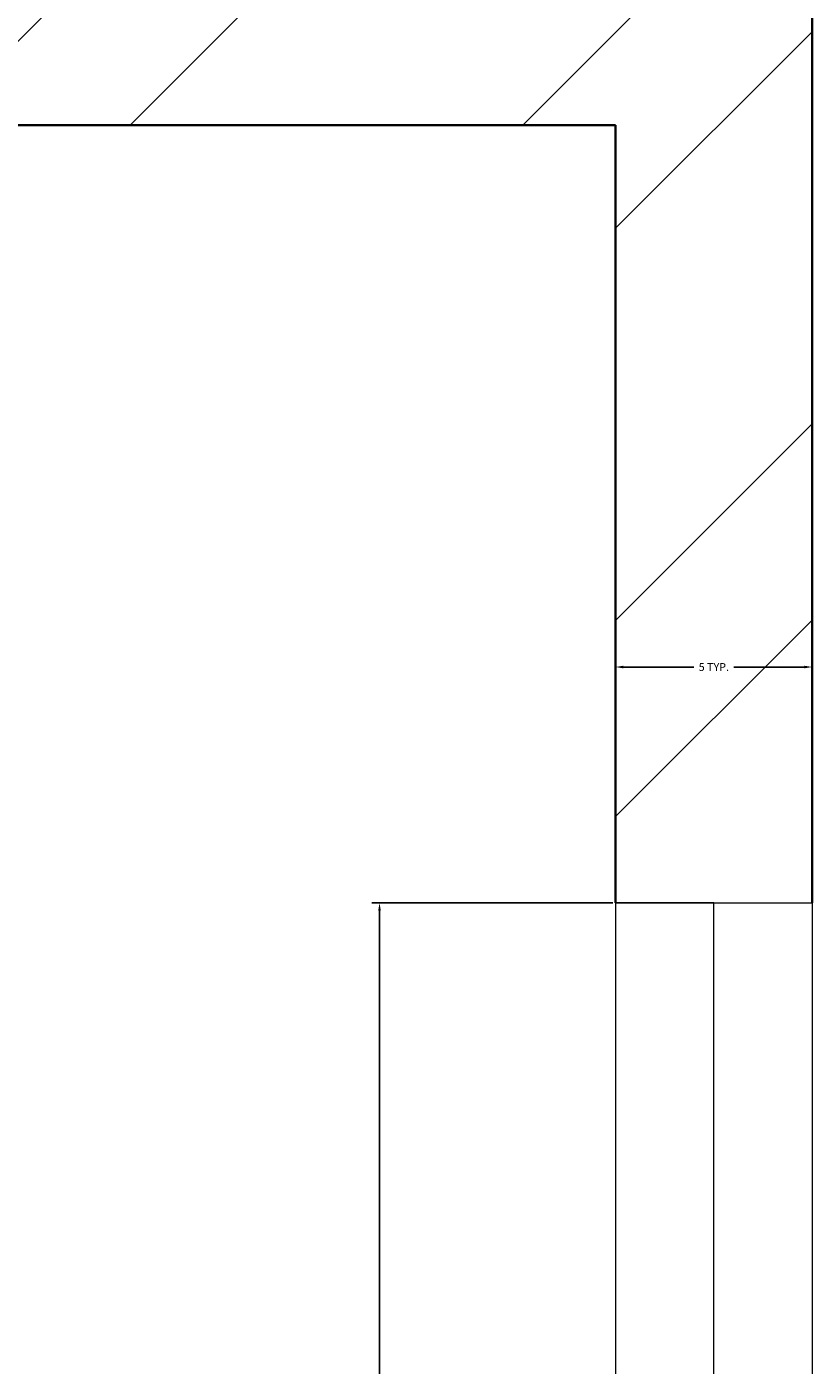
# Model space of a CAD drawing. Units: inches. Extents: x 2168 to 3056, y 1130 to 2629.
# Tile 20 of 42: x 2846 to 2864, y 2048 to 2079. Entities that reach past the tile are written whole.
import ezdxf

# ---------------------------------------------------------------- set-up
doc = ezdxf.new("R2010")
doc.units = ezdxf.units.IN
for name, color, linetype, lineweight in [('A-ANNO-DIMS', 2, 'Continuous', 18), ('A-GLAZ', 201, 'Continuous', 18), ('A-WALL', 7, 'Continuous', 35)]:
    doc.layers.add(name, color=color, linetype=linetype, lineweight=lineweight)
doc.layers.add('A-WALL-PATT', color=143, linetype='Continuous', lineweight=13, true_color=0x7aafdf)
doc.styles.get("Standard").update_dxf_attribs({"font": 'arial.ttf'})
doc.dimstyles.get("Standard").update_dxf_attribs({"dimtxt": 0.18, "dimasz": 0.18, "dimexe": 0.18, "dimexo": 0.0625, "dimgap": 0.09, "dimtad": 0, "dimtih": 1, "dimtoh": 1, "dimdec": 4, "dimzin": 0, "dimdsep": 46, "dimtxsty": 'Standard', "dimcen": 0.09, "dimadec": 0, "dimazin": 0, "dimtfac": 1, "dimtdec": 4, "dimtofl": 0, "dimtmove": 0, "dimatfit": 3, "dimfxl": 1, "dimtolj": 1, "dimtzin": 0, "dimarcsym": 0})

# ---------------------------------------------------------------- blocks, each defined once
blk = doc.blocks.new('WIN-36')
for p, q in [((2.25, 36), (0, 36)), ((0, 36), (4.5, 36)), ((0, 36), (0, 0)), ((2.25, 0), (2.25, 36)), ((4.5, 36), (4.5, 0))]:
    blk.add_line(p, q)
blk = doc.blocks.new('*D36')
at = {"layer": 'A-ANNO-DIMS', "color": 0, "lineweight": -2, "transparency": 16777216}
for p, q in [((2859.733, 2058.577), (2854.216, 2058.577)), ((2854.396, 2058.397), (2854.396, 2040.761)), ((2854.396, 2022.757), (2854.396, 2040.394)), ((2859.733, 2022.577), (2854.216, 2022.577))]:
    blk.add_line(p, q, dxfattribs=at)
at = {"layer": 'A-ANNO-DIMS', "color": 0, "transparency": 16777216}
for points in [[(2854.366, 2058.397), (2854.426, 2058.397), (2854.396, 2058.577)], [(2854.366, 2022.757), (2854.426, 2022.757), (2854.396, 2022.577)]]:
    blk.add_solid(points, dxfattribs=at)
at = {"layer": 'Defpoints', "color": 0, "transparency": 16777216}
for p in [(2854.396, 2058.577), (2859.796, 2058.577), (2859.796, 2022.577)]:
    blk.add_point(p, dxfattribs=at)
at = {"layer": 'A-ANNO-DIMS', "color": 0, "transparency": 16777216, "insert": (2854.396, 2040.577), "char_height": 0.18, "attachment_point": 5}
blk.add_mtext('\\A1;WINDOW 36 TYP.', dxfattribs=at)
blk = doc.blocks.new('*D37')
at = {"layer": 'A-ANNO-DIMS', "color": 0, "lineweight": -2, "transparency": 16777216}
for p, q in [((2859.796, 2058.64), (2859.796, 2064.157)), ((2864.296, 2058.64), (2864.296, 2064.157)), ((2859.976, 2063.977), (2861.588, 2063.977)), ((2864.116, 2063.977), (2862.504, 2063.977))]:
    blk.add_line(p, q, dxfattribs=at)
at = {"layer": 'A-ANNO-DIMS', "color": 0, "transparency": 16777216}
for points in [[(2859.976, 2064.007), (2859.976, 2063.947), (2859.796, 2063.977)], [(2864.116, 2064.007), (2864.116, 2063.947), (2864.296, 2063.977)]]:
    blk.add_solid(points, dxfattribs=at)
at = {"layer": 'Defpoints', "color": 0, "transparency": 16777216}
for p in [(2864.296, 2063.977), (2859.796, 2058.577), (2864.296, 2058.577)]:
    blk.add_point(p, dxfattribs=at)
at = {"layer": 'A-ANNO-DIMS', "color": 0, "transparency": 16777216, "insert": (2862.046, 2063.977), "char_height": 0.18, "attachment_point": 5}
blk.add_mtext('\\A1;5 TYP.', dxfattribs=at)

msp = doc.modelspace()

# ---------------------------------------------------------------- hatches: boundary and pattern name
at = {"layer": 'A-WALL-PATT'}
h = msp.add_hatch(dxfattribs=at)
h.set_pattern_fill('ANSI32', color=256)
h.paths.add_polyline_path([(2463.796, 2409.389), (2467.387, 2409.389), (2467.387, 2413.889), (2454.768, 2413.889), (2454.768, 2411.639), (2454.768, 2409.389), (2459.296, 2409.389), (2459.296, 2265.389), (2455.644, 2265.389), (2455.644, 2260.889), (2467.349, 2260.889), (2467.349, 2263.139), (2467.349, 2265.389), (2463.796, 2265.389)])
h.paths.add_polyline_path([(2431.596, 2413.889), (2409.647, 2413.889), (2409.647, 2409.389), (2431.596, 2409.389), (2431.596, 2411.639)])
h.paths.add_polyline_path([(2349.647, 2413.889), (2331.796, 2413.889), (2331.796, 2362.671), (2336.296, 2362.671), (2336.296, 2409.389), (2349.647, 2409.389), (2349.647, 2411.639)])
h.paths.add_polyline_path([(2634.149, 2411.639), (2634.149, 2413.889), (2562.293, 2413.889), (2562.293, 2409.389), (2595.796, 2409.389), (2595.796, 2280.309), (2595.826, 2280.309), (2595.826, 2265.389), (2499.91, 2265.389), (2499.91, 2260.889), (2550.796, 2260.889), (2550.796, 2117.308), (2555.296, 2117.308), (2555.296, 2168.08), (2571.93, 2168.08), (2571.93, 2176.889), (2559.796, 2176.889), (2559.796, 2256.389), (2640.796, 2256.389), (2640.796, 2176.889), (2626.428, 2176.889), (2626.428, 2168.08), (2645.296, 2168.08), (2645.296, 2116.637), (2649.796, 2116.637), (2649.796, 2260.889), (2691.251, 2260.889), (2691.251, 2263.139), (2691.251, 2265.389), (2670.655, 2265.389), (2670.655, 2265.365), (2600.296, 2265.365), (2600.296, 2280.258), (2600.296, 2409.389), (2634.149, 2409.389)])
h.paths.add_polyline_path([(2600.296, 2473.889), (2612.84, 2473.889), (2612.84, 2478.389), (2572.636, 2478.389), (2572.636, 2473.889), (2595.796, 2473.889), (2595.796, 2413.889), (2600.296, 2413.889)])
h.paths.add_polyline_path([(2535.796, 2473.889), (2548.636, 2473.889), (2548.636, 2478.389), (2531.396, 2478.389), (2531.396, 2413.889), (2521.6, 2413.889), (2521.6, 2409.389), (2539.239, 2409.389), (2539.239, 2411.639), (2539.239, 2413.889), (2535.796, 2413.889)])
h.paths.add_polyline_path([(2664.796, 2478.389), (2636.84, 2478.389), (2636.84, 2473.889), (2660.296, 2473.889), (2660.296, 2413.889), (2656.165, 2413.889), (2656.165, 2409.389), (2671.684, 2409.389), (2671.684, 2411.639), (2671.684, 2413.889), (2664.796, 2413.889)])
h.paths.add_polyline_path([(2705.942, 2413.889), (2695.684, 2413.889), (2695.684, 2409.389), (2705.942, 2409.389)])
h.paths.add_polyline_path([(2741.35, 2413.889), (2728.733, 2413.889), (2728.733, 2411.639), (2728.733, 2409.389), (2732.296, 2409.389), (2732.296, 2265.389), (2725.733, 2265.389), (2725.733, 2260.889), (2740.917, 2260.889), (2740.917, 2263.139), (2740.917, 2265.389), (2736.796, 2265.389), (2736.796, 2409.389), (2741.35, 2409.389)])
h.paths.add_polyline_path([(2785.655, 2413.889), (2764.546, 2413.889), (2764.486, 2409.389), (2785.655, 2409.389), (2785.655, 2411.639)])
h.paths.add_polyline_path([(2864.296, 2413.889), (2845.655, 2413.889), (2845.655, 2409.389), (2859.796, 2409.389), (2859.796, 2368.425), (2864.296, 2368.425)])
h.paths.add_polyline_path([(2864.296, 2308.425), (2862.046, 2308.425), (2859.796, 2308.425), (2859.796, 2265.389), (2774.483, 2265.389), (2774.483, 2263.139), (2774.483, 2260.889), (2781.796, 2260.889), (2781.796, 2226.654), (2786.296, 2226.654), (2786.296, 2260.889), (2859.796, 2260.889), (2859.796, 2241.352), (2864.296, 2241.352)])
h.paths.add_polyline_path([(2864.296, 2217.352), (2862.046, 2217.352), (2859.796, 2217.352), (2859.796, 2200.889), (2786.296, 2200.889), (2786.296, 2205.931), (2784.046, 2205.931), (2781.796, 2205.931), (2781.796, 2150.974), (2786.296, 2150.974), (2786.296, 2161.889), (2859.796, 2161.889), (2859.796, 2144.419), (2864.296, 2144.419)])
h.paths.add_polyline_path([(2859.796, 2196.389), (2859.796, 2166.389), (2786.296, 2166.389), (2786.296, 2196.389)], flags=16)
h.paths.add_polyline_path([(2864.296, 2108.419), (2862.046, 2108.419), (2859.796, 2108.419), (2859.796, 2080.889), (2786.296, 2080.889), (2786.296, 2111.993), (2781.796, 2111.993), (2781.796, 2080.889), (2649.796, 2080.889), (2649.796, 2086.036), (2647.546, 2086.036), (2645.296, 2086.036), (2645.296, 2071.739), (2649.796, 2071.739), (2649.796, 2076.389), (2781.796, 2076.389), (2781.796, 2041.792), (2786.296, 2041.792), (2786.296, 2076.389), (2859.796, 2076.389), (2859.796, 2058.577), (2864.296, 2058.577)])
h.paths.add_polyline_path([(2864.296, 2022.577), (2859.796, 2022.577), (2859.796, 1992.389), (2786.296, 1992.389), (2786.296, 1999.573), (2781.796, 1999.573), (2781.796, 1848.085), (2784.046, 1848.085), (2786.296, 1848.085), (2786.296, 1851.389), (2859.796, 1851.389), (2859.796, 1838.258), (2864.296, 1838.258)], flags=17)
h.paths.add_polyline_path([(2859.796, 1987.889), (2859.796, 1855.889), (2786.296, 1855.889), (2786.296, 1987.889)], flags=16)
h.paths.add_polyline_path([(2823.046, 1987.889), (2841.421, 1921.889), (2823.046, 1855.889)], flags=0)
h.paths.add_polyline_path([(2864.296, 1814.258), (2859.796, 1814.258), (2859.796, 1791.389), (2786.296, 1791.389), (2786.296, 1825.658), (2784.046, 1825.658), (2781.796, 1825.658), (2781.796, 1791.389), (2720.155, 1791.389), (2720.155, 1791.265), (2649.796, 1791.265), (2649.796, 1806.159), (2649.796, 2038.983), (2647.546, 2038.983), (2645.296, 2038.983), (2645.296, 1783.925), (2649.796, 1783.925), (2649.796, 1786.889), (2781.796, 1786.889), (2781.796, 1746.789), (2786.296, 1746.789), (2786.296, 1786.889), (2859.796, 1786.889), (2859.796, 1770.083), (2864.296, 1770.083)])
h.paths.add_polyline_path([(2864.296, 1734.083), (2862.046, 1734.083), (2859.796, 1734.083), (2859.796, 1705.889), (2786.296, 1705.889), (2786.296, 1714.166), (2781.796, 1714.166), (2781.796, 1660.527), (2786.296, 1660.527), (2786.296, 1666.889), (2859.796, 1666.889), (2859.796, 1648.342), (2864.296, 1648.342)])
h.paths.add_polyline_path([(2786.296, 1701.389), (2859.796, 1701.389), (2859.796, 1671.389), (2786.296, 1671.389)], flags=16)
h.paths.add_polyline_path([(2649.796, 1756.576), (2647.546, 1756.576), (2645.296, 1756.576), (2645.296, 1606.889), (2555.296, 1606.889), (2555.296, 1749.513), (2553.046, 1749.513), (2550.796, 1749.513), (2550.796, 1606.889), (2503.006, 1606.889), (2503.006, 1604.639), (2503.006, 1602.389), (2595.796, 1602.389), (2595.849, 1602.389), (2595.849, 1587.495), (2595.796, 1458.389), (2561.502, 1458.389), (2561.502, 1456.139), (2561.502, 1453.889), (2595.796, 1453.889), (2595.796, 1381.889), (2573.438, 1381.889), (2573.438, 1377.389), (2613.01, 1377.389), (2613.01, 1379.639), (2613.01, 1381.889), (2600.296, 1381.889), (2600.296, 1453.889), (2634.327, 1453.889), (2634.327, 1458.389), (2600.296, 1458.389), (2600.296, 1602.389), (2670.655, 1602.389), (2694.095, 1602.389), (2694.095, 1606.889), (2649.796, 1606.889)])
h.paths.add_polyline_path([(2736.796, 1602.389), (2741.562, 1602.389), (2741.562, 1606.889), (2726.203, 1606.889), (2726.203, 1604.639), (2726.203, 1602.389), (2732.296, 1602.389), (2732.296, 1458.389), (2727.899, 1458.389), (2727.899, 1453.889), (2740.821, 1453.889), (2740.821, 1456.139), (2740.821, 1458.389), (2736.796, 1458.389)])
h.paths.add_polyline_path([(2859.796, 1606.889), (2786.296, 1606.889), (2786.296, 1637.334), (2784.046, 1637.334), (2781.796, 1637.334), (2781.796, 1606.889), (2775.612, 1606.889), (2775.612, 1602.389), (2859.796, 1602.389)])
h.paths.add_polyline_path([(2864.296, 1624.342), (2862.046, 1624.342), (2859.796, 1624.342), (2859.796, 1570.39), (2864.296, 1570.39)])
h.paths.add_polyline_path([(2864.296, 1510.39), (2862.046, 1510.39), (2859.796, 1510.39), (2859.796, 1458.389), (2846.735, 1458.389), (2846.735, 1456.139), (2846.735, 1453.889), (2864.296, 1453.889)])
h.paths.add_polyline_path([(2786.735, 1458.389), (2765.444, 1458.389), (2765.444, 1453.889), (2786.735, 1453.889)])
h.paths.add_polyline_path([(2706.004, 1458.389), (2695.36, 1458.389), (2695.36, 1453.889), (2706.004, 1453.889), (2706.004, 1456.139)])
h.paths.add_polyline_path([(2671.36, 1456.139), (2671.36, 1458.389), (2655.986, 1458.389), (2655.986, 1456.139), (2655.986, 1453.889), (2660.296, 1453.889), (2660.296, 1381.889), (2637.01, 1381.889), (2637.01, 1377.389), (2664.796, 1377.389), (2664.796, 1453.889), (2671.36, 1453.889)], flags=17)
h.paths.add_polyline_path([(2539.829, 1458.389), (2520.237, 1458.389), (2520.237, 1453.889), (2531.296, 1453.889), (2531.296, 1377.389), (2546.449, 1377.389), (2546.449, 1379.639), (2546.449, 1381.889), (2535.796, 1381.889), (2535.796, 1453.889), (2539.829, 1453.889)], flags=17)
h.paths.add_polyline_path([(2496.237, 1458.389), (2489.13, 1458.389), (2489.13, 1453.889), (2496.237, 1453.889), (2496.237, 1456.139)])
h.paths.add_polyline_path([(2467.433, 1456.139), (2467.433, 1458.389), (2463.796, 1458.389), (2463.796, 1602.389), (2468.242, 1602.389), (2468.242, 1605.7), (2468.242, 1606.889), (2454.602, 1606.889), (2454.602, 1602.389), (2459.296, 1602.389), (2459.296, 1458.389), (2454.24, 1458.389), (2454.24, 1453.889), (2467.433, 1453.889)])
h.paths.add_polyline_path([(2431.601, 1456.139), (2431.601, 1458.389), (2411.386, 1458.389), (2411.386, 1453.889), (2431.601, 1453.889)])
h.paths.add_polyline_path([(2351.386, 1458.389), (2336.296, 1458.389), (2336.296, 1490.693), (2334.046, 1490.693), (2331.796, 1490.693), (2331.796, 1453.889), (2351.386, 1453.889), (2351.386, 1456.139)])
h.paths.add_polyline_path([(2336.296, 1629.705), (2331.796, 1629.705), (2331.796, 1552.317), (2336.296, 1552.317), (2336.296, 1602.389), (2406.655, 1602.389), (2423.472, 1602.389), (2423.472, 1606.889), (2418.796, 1606.889), (2418.796, 1643.678), (2416.546, 1643.678), (2414.296, 1643.678), (2414.296, 1606.889), (2336.296, 1606.889)])
h.paths.add_polyline_path([(2418.796, 1714.384), (2414.296, 1714.384), (2414.296, 1705.889), (2336.296, 1705.889), (2336.296, 1731.324), (2334.046, 1731.324), (2331.796, 1731.324), (2331.796, 1653.705), (2334.046, 1653.705), (2336.296, 1653.705), (2336.296, 1666.889), (2414.296, 1666.889), (2414.296, 1663.589), (2418.796, 1663.589)])
h.paths.add_polyline_path([(2336.296, 1701.389), (2414.296, 1701.389), (2414.296, 1671.389), (2336.296, 1671.389)], flags=16)
h.paths.add_polyline_path([(2555.296, 2040.059), (2550.796, 2040.059), (2550.796, 1791.389), (2550.561, 1791.205), (2480.202, 1791.205), (2418.796, 1791.389), (2418.796, 1825.448), (2416.546, 1825.448), (2414.296, 1825.448), (2414.296, 1791.389), (2336.296, 1791.389), (2336.296, 1806.409), (2331.796, 1806.409), (2331.796, 1767.324), (2336.296, 1767.324), (2336.296, 1786.889), (2414.296, 1786.889), (2414.296, 1745.457), (2418.796, 1745.457), (2418.796, 1786.889), (2550.796, 1786.889), (2550.796, 1783.011), (2555.296, 1783.011)])
h.paths.add_polyline_path([(2418.796, 1923.389), (2423.207, 1923.389), (2423.207, 1925.639), (2423.207, 1927.889), (2418.796, 1927.889), (2418.796, 2000.048), (2414.296, 2000.048), (2414.296, 1992.389), (2336.296, 1992.389), (2336.296, 1987.889), (2414.296, 1987.889), (2414.296, 1855.889), (2336.296, 1855.889), (2336.296, 1851.389), (2414.296, 1851.389), (2414.296, 1846.759), (2418.796, 1846.759)], flags=17)
h.paths.add_polyline_path([(2336.296, 2019.294), (2334.046, 2019.294), (2331.796, 2019.294), (2331.796, 1830.409), (2336.296, 1830.409)], flags=17)
h.paths.add_polyline_path([(2550.796, 1927.889), (2453.541, 1927.889), (2453.541, 1925.639), (2453.541, 1923.389), (2550.796, 1923.389)], flags=17)
h.paths.add_polyline_path([(2744.987, 1927.889), (2649.796, 1927.889), (2649.796, 1923.389), (2744.987, 1923.389), (2744.987, 1925.639)], flags=17)
h.paths.add_polyline_path([(2555.296, 2086.458), (2553.046, 2086.458), (2550.796, 2086.458), (2550.796, 2080.889), (2418.796, 2080.889), (2336.296, 2080.889), (2336.296, 2115.399), (2334.046, 2115.399), (2331.796, 2115.399), (2331.796, 2055.294), (2336.296, 2055.294), (2336.296, 2076.389), (2550.796, 2076.389), (2550.796, 2071.538), (2555.296, 2071.538)])
h.paths.add_polyline_path([(2418.796, 2121.389), (2414.296, 2121.389), (2414.296, 2080.889), (2418.796, 2080.889)])
h.paths.add_polyline_path([(2418.796, 2076.389), (2414.296, 2076.389), (2414.296, 2035.123), (2418.796, 2035.123)])
h.paths.add_polyline_path([(2422.868, 2263.139), (2422.868, 2265.389), (2406.655, 2265.389), (2406.655, 2265.359), (2336.296, 2265.359), (2336.296, 2280.252), (2336.296, 2302.671), (2334.046, 2302.671), (2331.796, 2302.671), (2331.796, 2246.853), (2336.296, 2246.853), (2336.296, 2260.889), (2414.296, 2260.889), (2414.296, 2223.996), (2418.796, 2223.996), (2418.796, 2260.889), (2422.868, 2260.889)])
h.paths.add_polyline_path([(2418.796, 2204.783), (2416.546, 2204.783), (2414.296, 2204.783), (2414.296, 2200.889), (2336.296, 2200.889), (2336.296, 2220.853), (2331.796, 2220.853), (2331.796, 2151.399), (2336.296, 2151.399), (2336.296, 2161.889), (2414.296, 2161.889), (2414.296, 2153.726), (2418.796, 2153.726)])
h.paths.add_polyline_path([(2414.296, 2196.389), (2414.296, 2166.389), (2336.296, 2166.389), (2336.296, 2196.389)], flags=16)
h.paths.add_polyline_path([(2375.296, 2181.389), (2336.296, 2166.389), (2336.296, 2196.389)], flags=0)
h.paths.add_polyline_path([(2809.595, 2172.34), (2838.804, 2172.34), (2838.804, 2190.997), (2809.595, 2190.997)], flags=8)
h.paths.add_polyline_path([(2849.75, 1919.585), (2849.75, 1952.672), (2831.093, 1952.672), (2831.093, 1919.585)], flags=8)
h.paths.add_polyline_path([(2808.875, 1901.967), (2808.875, 1937.85), (2790.149, 1937.85), (2790.149, 1901.967)], flags=8)
h.paths.add_polyline_path([(2806.285, 1671.896), (2835.493, 1671.896), (2835.493, 1690.553), (2806.285, 1690.553)], flags=8)
h.paths.add_polyline_path([(2353.186, 1676.549), (2382.395, 1676.549), (2382.395, 1695.207), (2353.186, 1695.207)], flags=8)
h.paths.add_polyline_path([(2360.083, 1832.308), (2389.241, 1832.308), (2389.241, 1850.966), (2360.083, 1850.966)], flags=25)
h.paths.add_polyline_path([(2354.822, 2167.823), (2384.031, 2167.823), (2384.031, 2186.481), (2354.822, 2186.481)], flags=8)

# ---------------------------------------------------------------- linework, layer by layer
at = {"layer": 'A-GLAZ'}
msp.add_line((2859.796, 2058.577), (2859.796, 2058.577), dxfattribs=at)
at = {"layer": 'A-WALL'}
for p, q in [((2864.296, 2108.419), (2864.296, 2058.577)), ((2786.296, 2076.389), (2859.796, 2076.389)), ((2859.796, 2076.389), (2859.796, 2058.577))]:
    msp.add_line(p, q, dxfattribs=at)

# ---------------------------------------------------------------- block references
at = {"layer": 'A-GLAZ'}
msp.add_blockref('WIN-36', (2859.796, 2022.578), dxfattribs=at)

# ---------------------------------------------------------------- dimensions: what is measured, and where the dimension line sits
at = {"layer": 'A-ANNO-DIMS'}
dim = msp.add_linear_dim(base=(2864.29575579, 2063.977351816), p1=(2859.79575579, 2058.577351816), p2=(2864.29575579, 2058.577351816), text='<> TYP.', dimstyle='Standard', override={"dimdec": 0, "dimlfac": 1, "dimrnd": 0, "dimzin": 0, "dimdsep": 46, "dimlunit": 2}, dxfattribs=at)
dim.commit()
dim.dimension.update_dxf_attribs({"geometry": '*D37', "text_midpoint": (2862.04575579, 2063.977351816)})
dim = msp.add_linear_dim(base=(2854.396, 2058.577), p1=(2859.796, 2022.577), p2=(2859.796, 2058.577), angle=90, text='WINDOW <> TYP.', dimstyle='Standard', override={"dimdec": 0, "dimlfac": 1, "dimrnd": 0, "dimzin": 0, "dimdsep": 46, "dimlunit": 2}, dxfattribs=at)
dim.commit()
dim.dimension.update_dxf_attribs({"geometry": '*D36', "text_midpoint": (2854.396, 2040.577)})

doc.saveas('drawing.dxf')
